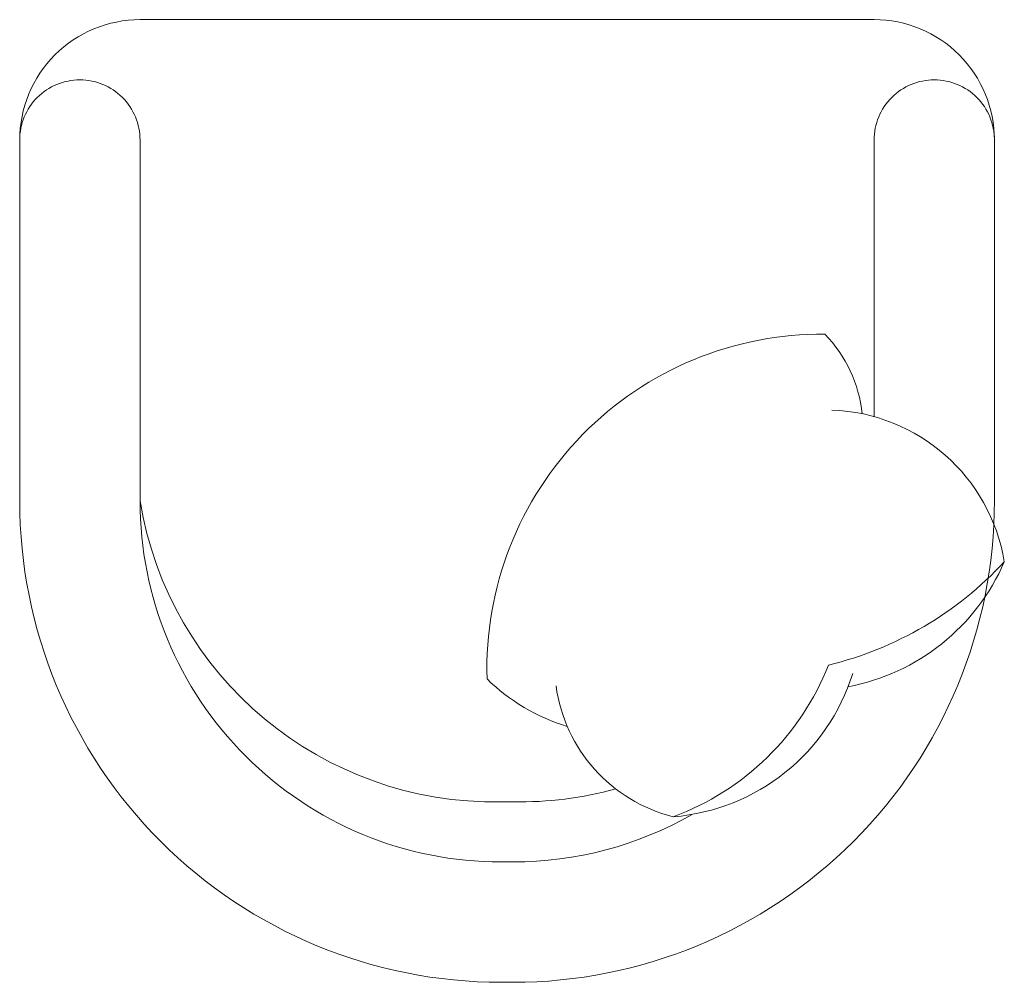
# Model space of a CAD drawing. Units: inches. Extents: x 963 to 2075, y 289 to 2657.
# Tile 19 of 98: x 1467 to 1484, y 1732 to 1749. Entities that reach past the tile are written whole.
import ezdxf

# ---------------------------------------------------------------- set-up
doc = ezdxf.new("R2010")
doc.units = ezdxf.units.IN
doc.layers.add('A-FURN', color=8, linetype='Continuous', lineweight=18)

msp = doc.modelspace()

# ---------------------------------------------------------------- linework, layer by layer
at = {"layer": 'A-FURN', "ltscale": 0.03}
msp.add_lwpolyline([(1475.609, 1748.968), (1469.235, 1748.968, 0.414214), (1467.146, 1746.878), (1467.146, 1740.609, 0.414214), (1475.504, 1732.25), (1475.609, 1732.25), (1475.713, 1732.25, 0.414214), (1484.072, 1740.609), (1484.072, 1746.878, 0.414214), (1481.982, 1748.968), (1475.609, 1748.968)], format="xyb", dxfattribs=at)
at = {"layer": 'A-FURN'}
for points in [[(1469.235, 1740.609), (1469.235, 1746.878, 0.414214), (1468.191, 1747.923), (1468.191, 1747.923, 0.414214), (1467.146, 1746.878)], [(1481.982, 1742.074), (1481.982, 1746.878, -0.414214), (1483.027, 1747.923), (1483.027, 1747.923, -0.414214), (1484.072, 1746.878)], [(1481.776, 1742.124, 0.165541), (1481.129, 1743.505, 0.425989), (1475.261, 1737.519, 0.121523), (1476.654, 1736.694, -7.115464)], [(1481.249, 1742.188, -0.356772), (1484.243, 1739.554, -0.249542), (1481.53, 1737.384, 9.61688)], [(1469.235, 1740.609, 0.372719), (1475.504, 1735.385), (1475.609, 1735.385)], [(1469.235, 1740.609, 0.414214), (1475.504, 1734.34), (1475.609, 1734.34)], [(1484.243, 1739.554, -0.14773), (1481.189, 1737.759, -0.213343), (1478.495, 1735.125, -0.178662)], [(1481.611, 1737.615, -0.306663), (1478.495, 1735.125, -0.30633), (1476.459, 1737.399, 0.872847)], [(1477.495, 1735.61, -0.072384), (1475.713, 1735.385), (1475.609, 1735.385)], [(1478.825, 1735.167, -0.130591), (1475.713, 1734.34), (1475.609, 1734.34)]]:
    msp.add_lwpolyline(points, format="xyb", dxfattribs=at)

doc.saveas('drawing.dxf')
